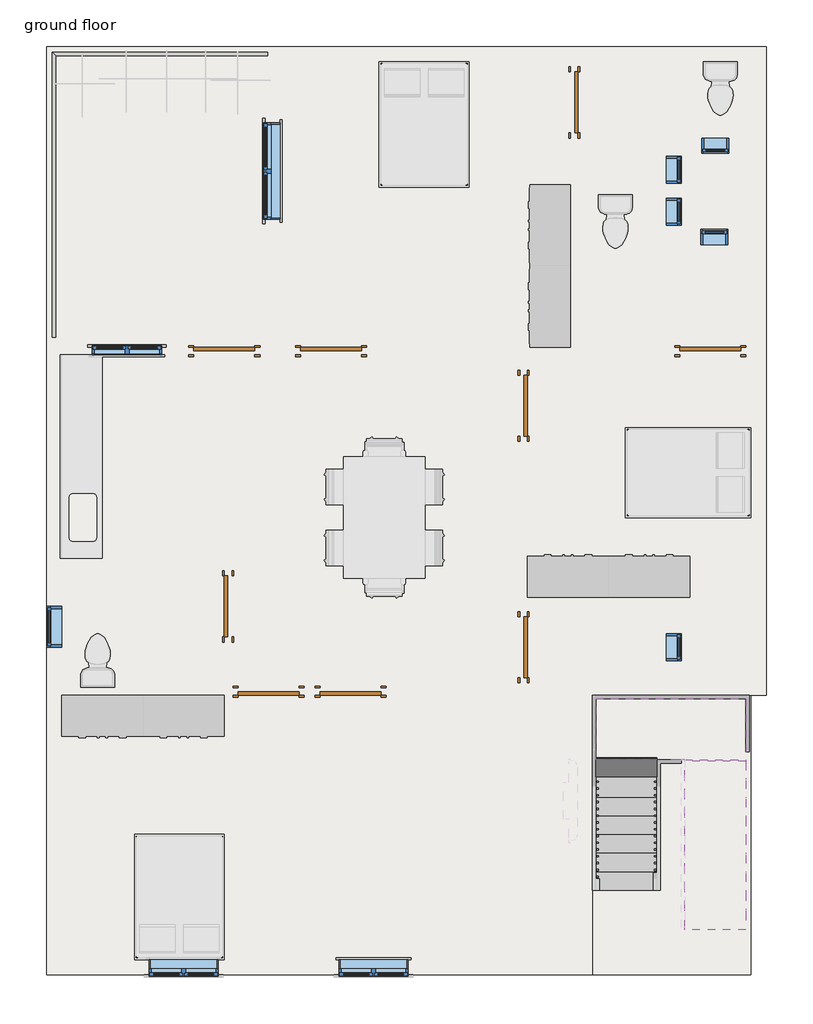
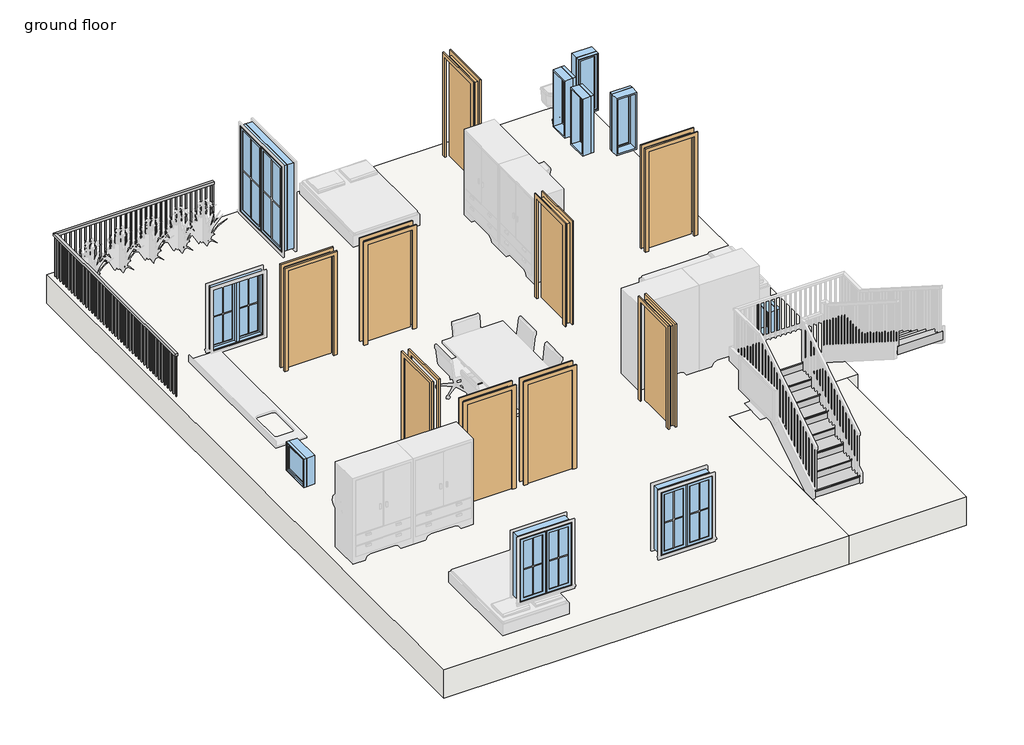
# One storey, part 1 of 3: 10 windows, 9 doors, 3 slabs, 2 stair flights, 1 railing.
"""IFC4 building model written with IfcOpenShell, lengths in millimetres."""

from ifc_helpers import new_model, si_unit, frame, origin, origin_with_axes, place, context, project, spatial, polyline, outline, extrude, faceted_brep, transform, mapped, element, save
from components import door_305aa2a5, door_e5f9f3c4, non_monolithic_landing_cf1353f8, stair_flight_d2e0b81c, stair_flight_50bec54b, window_aa618e30, window_cea7027f, window_80340324, window_8ddb865a, window_c95ebb39, window_9ac97e1a

model = new_model("IFC4")

# Units and contexts
model_context = context("Model", 3, world=origin())
ifc_project = project(units=[si_unit("LENGTHUNIT", "METRE", prefix="MILLI")], contexts=[model_context])

# Site, building, storey
site = spatial("IfcSite", under=ifc_project)
building = spatial("IfcBuilding", under=site)
storey = spatial("IfcBuildingStorey", under=building, Name="ground floor", Elevation=609.6)

# Doors
placement = place(None, origin())
door_shape = door_305aa2a5(model_context)
element("IfcDoor", 1, ObjectType="Single-Flush : 36\" x 84\"", at=placement, inside=storey, context=model_context, shape_type="MappedRepresentation", body=[
    mapped(door_shape, transform((-191.8998597, 11968.6257925, 609.6), x_axis=(0.0, 1.0, 0.0), y_axis=(-1.0, 0.0, 0.0), z_axis=(0.0, 0.0, 1.0))),
])
element("IfcDoor", 2, ObjectType="Single-Flush : 36\" x 84\"", at=placement, inside=storey, context=model_context, shape_type="MappedRepresentation", body=[
    mapped(door_shape, transform((-3843.1498597, 8241.1757925, 609.6), x_axis=(-1.0, 0.0, 0.0), y_axis=(0.0, -1.0, 0.0), z_axis=(0.0, 0.0, 1.0))),
])
element("IfcDoor", 3, ObjectType="Single-Flush : 36\" x 84\"", at=placement, inside=storey, context=model_context, shape_type="MappedRepresentation", body=[
    mapped(door_shape, transform((-953.8998597, 7422.0257925, 609.6), x_axis=(0.0, 1.0, 0.0), y_axis=(-1.0, 0.0, 0.0), z_axis=(0.0, 0.0, 1.0))),
])
element("IfcDoor", 4, ObjectType="Single-Flush : 36\" x 84\"", at=placement, inside=storey, context=model_context, shape_type="MappedRepresentation", body=[
    mapped(door_shape, transform((-4776.5998597, 3135.7757925, 609.6), x_axis=(1.0, 0.0, 0.0), y_axis=(0.0, 1.0, 0.0), z_axis=(0.0, 0.0, 1.0))),
])
door_2_shape = door_e5f9f3c4(model_context)
element("IfcDoor", 5, ObjectType="Single-Flush : 36\" x 84\"", at=placement, inside=storey, context=model_context, shape_type="MappedRepresentation", body=[
    mapped(door_2_shape, transform((1846.4501403, 8241.1757925, 609.6), x_axis=(1.0, 0.0, 0.0), y_axis=(0.0, 1.0, 0.0), z_axis=(0.0, 0.0, 1.0))),
])
element("IfcDoor", 6, ObjectType="Single-Flush : 36\" x 84\"", at=placement, inside=storey, context=model_context, shape_type="MappedRepresentation", body=[
    mapped(door_2_shape, transform((-5386.1998597, 4412.1257925, 609.6), x_axis=(0.0, 1.0, 0.0), y_axis=(-1.0, 0.0, 0.0), z_axis=(0.0, 0.0, 1.0))),
])
element("IfcDoor", 7, ObjectType="Single-Flush : 36\" x 84\"", at=placement, inside=storey, context=model_context, shape_type="MappedRepresentation", body=[
    mapped(door_2_shape, transform((-3551.0498597, 3135.7757925, 609.6), x_axis=(-1.0, 0.0, 0.0), y_axis=(0.0, -1.0, 0.0), z_axis=(0.0, 0.0, 1.0))),
])
element("IfcDoor", 8, ObjectType="Single-Flush : 36\" x 84\"", at=placement, inside=storey, context=model_context, shape_type="MappedRepresentation", body=[
    mapped(door_2_shape, transform((-953.8998597, 3802.5257925, 609.6), x_axis=(0.0, -1.0, 0.0), y_axis=(1.0, 0.0, 0.0), z_axis=(0.0, 0.0, 1.0))),
])
element("IfcDoor", 9, ObjectType="Single-Flush : 36\" x 84\"", at=placement, inside=storey, context=model_context, shape_type="MappedRepresentation", body=[
    mapped(door_2_shape, transform((-5443.3498597, 8241.1757925, 609.6), x_axis=(1.0, 0.0, 0.0), y_axis=(0.0, 1.0, 0.0), z_axis=(0.0, 0.0, 1.0))),
])

# Railing
element("IfcRailing", 10, ObjectType="Handrail - Rectangular", at=placement, inside=storey, context=model_context, shape_type="SolidModel", body=[
    faceted_brep([(-8021.4498597, 8450.7257925, 1524.0), (-8021.4498597, 8450.7257925, 1473.2), (-7970.6498597, 8450.7257925, 1473.2), (-7970.6498597, 8450.7257925, 1524.0), (-8021.4498597, 12717.9257925, 1524.0), (-8021.4498597, 12717.9257925, 1473.2), (-7970.6498597, 12667.1257925, 1473.2), (-7970.6498597, 12667.1257925, 1524.0), (-4795.6498597, 12717.9257925, 1524.0), (-4795.6498597, 12667.1257925, 1524.0), (-4795.6498597, 12667.1257925, 1473.2), (-4795.6498597, 12717.9257925, 1473.2)], [[[0, 1, 2, 3]], [[1, 0, 4, 5]], [[2, 1, 5, 6]], [[3, 2, 6, 7]], [[0, 3, 7, 4]], [[8, 9, 10, 11]], [[5, 4, 8, 11]], [[6, 5, 11, 10]], [[7, 6, 10, 9]], [[4, 7, 9, 8]]]),
    extrude(outline(polyline([(-4855.9748597, 12683.0007925), (-4855.9748597, 12702.0507925), (-4836.9248597, 12702.0507925), (-4836.9248597, 12683.0007925), (-4855.9748597, 12683.0007925)])), frame((0.0, 0.0, 609.6), z_axis=(0.0, 0.0, 1.0), x_axis=(1.0, 0.0, 0.0)), (0.0, 0.0, 1.0), 863.6),
    extrude(outline(polyline([(-4957.5748597, 12683.0007925), (-4957.5748597, 12702.0507925), (-4938.5248597, 12702.0507925), (-4938.5248597, 12683.0007925), (-4957.5748597, 12683.0007925)])), frame((0.0, 0.0, 609.6), z_axis=(0.0, 0.0, 1.0), x_axis=(1.0, 0.0, 0.0)), (0.0, 0.0, 1.0), 863.6),
    extrude(outline(polyline([(-5059.1748597, 12683.0007925), (-5059.1748597, 12702.0507925), (-5040.1248597, 12702.0507925), (-5040.1248597, 12683.0007925), (-5059.1748597, 12683.0007925)])), frame((0.0, 0.0, 609.6), z_axis=(0.0, 0.0, 1.0), x_axis=(1.0, 0.0, 0.0)), (0.0, 0.0, 1.0), 863.6),
    extrude(outline(polyline([(-5160.7748597, 12683.0007925), (-5160.7748597, 12702.0507925), (-5141.7248597, 12702.0507925), (-5141.7248597, 12683.0007925), (-5160.7748597, 12683.0007925)])), frame((0.0, 0.0, 609.6), z_axis=(0.0, 0.0, 1.0), x_axis=(1.0, 0.0, 0.0)), (0.0, 0.0, 1.0), 863.6),
    extrude(outline(polyline([(-5262.3748597, 12683.0007925), (-5262.3748597, 12702.0507925), (-5243.3248597, 12702.0507925), (-5243.3248597, 12683.0007925), (-5262.3748597, 12683.0007925)])), frame((0.0, 0.0, 609.6), z_axis=(0.0, 0.0, 1.0), x_axis=(1.0, 0.0, 0.0)), (0.0, 0.0, 1.0), 863.6),
    extrude(outline(polyline([(-5363.9748597, 12683.0007925), (-5363.9748597, 12702.0507925), (-5344.9248597, 12702.0507925), (-5344.9248597, 12683.0007925), (-5363.9748597, 12683.0007925)])), frame((0.0, 0.0, 609.6), z_axis=(0.0, 0.0, 1.0), x_axis=(1.0, 0.0, 0.0)), (0.0, 0.0, 1.0), 863.6),
    extrude(outline(polyline([(-5465.5748597, 12683.0007925), (-5465.5748597, 12702.0507925), (-5446.5248597, 12702.0507925), (-5446.5248597, 12683.0007925), (-5465.5748597, 12683.0007925)])), frame((0.0, 0.0, 609.6), z_axis=(0.0, 0.0, 1.0), x_axis=(1.0, 0.0, 0.0)), (0.0, 0.0, 1.0), 863.6),
    extrude(outline(polyline([(-5567.1748597, 12683.0007925), (-5567.1748597, 12702.0507925), (-5548.1248597, 12702.0507925), (-5548.1248597, 12683.0007925), (-5567.1748597, 12683.0007925)])), frame((0.0, 0.0, 609.6), z_axis=(0.0, 0.0, 1.0), x_axis=(1.0, 0.0, 0.0)), (0.0, 0.0, 1.0), 863.6),
    extrude(outline(polyline([(-5668.7748597, 12683.0007925), (-5668.7748597, 12702.0507925), (-5649.7248597, 12702.0507925), (-5649.7248597, 12683.0007925), (-5668.7748597, 12683.0007925)])), frame((0.0, 0.0, 609.6), z_axis=(0.0, 0.0, 1.0), x_axis=(1.0, 0.0, 0.0)), (0.0, 0.0, 1.0), 863.6),
    extrude(outline(polyline([(-5770.3748597, 12683.0007925), (-5770.3748597, 12702.0507925), (-5751.3248597, 12702.0507925), (-5751.3248597, 12683.0007925), (-5770.3748597, 12683.0007925)])), frame((0.0, 0.0, 609.6), z_axis=(0.0, 0.0, 1.0), x_axis=(1.0, 0.0, 0.0)), (0.0, 0.0, 1.0), 863.6),
    extrude(outline(polyline([(-5871.9748597, 12683.0007925), (-5871.9748597, 12702.0507925), (-5852.9248597, 12702.0507925), (-5852.9248597, 12683.0007925), (-5871.9748597, 12683.0007925)])), frame((0.0, 0.0, 609.6), z_axis=(0.0, 0.0, 1.0), x_axis=(1.0, 0.0, 0.0)), (0.0, 0.0, 1.0), 863.6),
    extrude(outline(polyline([(-5973.5748597, 12683.0007925), (-5973.5748597, 12702.0507925), (-5954.5248597, 12702.0507925), (-5954.5248597, 12683.0007925), (-5973.5748597, 12683.0007925)])), frame((0.0, 0.0, 609.6), z_axis=(0.0, 0.0, 1.0), x_axis=(1.0, 0.0, 0.0)), (0.0, 0.0, 1.0), 863.6),
    extrude(outline(polyline([(-6075.1748597, 12683.0007925), (-6075.1748597, 12702.0507925), (-6056.1248597, 12702.0507925), (-6056.1248597, 12683.0007925), (-6075.1748597, 12683.0007925)])), frame((0.0, 0.0, 609.6), z_axis=(0.0, 0.0, 1.0), x_axis=(1.0, 0.0, 0.0)), (0.0, 0.0, 1.0), 863.6),
    extrude(outline(polyline([(-6176.7748597, 12683.0007925), (-6176.7748597, 12702.0507925), (-6157.7248597, 12702.0507925), (-6157.7248597, 12683.0007925), (-6176.7748597, 12683.0007925)])), frame((0.0, 0.0, 609.6), z_axis=(0.0, 0.0, 1.0), x_axis=(1.0, 0.0, 0.0)), (0.0, 0.0, 1.0), 863.6),
    extrude(outline(polyline([(-6278.3748597, 12683.0007925), (-6278.3748597, 12702.0507925), (-6259.3248597, 12702.0507925), (-6259.3248597, 12683.0007925), (-6278.3748597, 12683.0007925)])), frame((0.0, 0.0, 609.6), z_axis=(0.0, 0.0, 1.0), x_axis=(1.0, 0.0, 0.0)), (0.0, 0.0, 1.0), 863.6),
    extrude(outline(polyline([(-6379.9748597, 12683.0007925), (-6379.9748597, 12702.0507925), (-6360.9248597, 12702.0507925), (-6360.9248597, 12683.0007925), (-6379.9748597, 12683.0007925)])), frame((0.0, 0.0, 609.6), z_axis=(0.0, 0.0, 1.0), x_axis=(1.0, 0.0, 0.0)), (0.0, 0.0, 1.0), 863.6),
    extrude(outline(polyline([(-6481.5748597, 12683.0007925), (-6481.5748597, 12702.0507925), (-6462.5248597, 12702.0507925), (-6462.5248597, 12683.0007925), (-6481.5748597, 12683.0007925)])), frame((0.0, 0.0, 609.6), z_axis=(0.0, 0.0, 1.0), x_axis=(1.0, 0.0, 0.0)), (0.0, 0.0, 1.0), 863.6),
    extrude(outline(polyline([(-6583.1748597, 12683.0007925), (-6583.1748597, 12702.0507925), (-6564.1248597, 12702.0507925), (-6564.1248597, 12683.0007925), (-6583.1748597, 12683.0007925)])), frame((0.0, 0.0, 609.6), z_axis=(0.0, 0.0, 1.0), x_axis=(1.0, 0.0, 0.0)), (0.0, 0.0, 1.0), 863.6),
    extrude(outline(polyline([(-6684.7748597, 12683.0007925), (-6684.7748597, 12702.0507925), (-6665.7248597, 12702.0507925), (-6665.7248597, 12683.0007925), (-6684.7748597, 12683.0007925)])), frame((0.0, 0.0, 609.6), z_axis=(0.0, 0.0, 1.0), x_axis=(1.0, 0.0, 0.0)), (0.0, 0.0, 1.0), 863.6),
    extrude(outline(polyline([(-6786.3748597, 12683.0007925), (-6786.3748597, 12702.0507925), (-6767.3248597, 12702.0507925), (-6767.3248597, 12683.0007925), (-6786.3748597, 12683.0007925)])), frame((0.0, 0.0, 609.6), z_axis=(0.0, 0.0, 1.0), x_axis=(1.0, 0.0, 0.0)), (0.0, 0.0, 1.0), 863.6),
    extrude(outline(polyline([(-6887.9748597, 12683.0007925), (-6887.9748597, 12702.0507925), (-6868.9248597, 12702.0507925), (-6868.9248597, 12683.0007925), (-6887.9748597, 12683.0007925)])), frame((0.0, 0.0, 609.6), z_axis=(0.0, 0.0, 1.0), x_axis=(1.0, 0.0, 0.0)), (0.0, 0.0, 1.0), 863.6),
    extrude(outline(polyline([(-6989.5748597, 12683.0007925), (-6989.5748597, 12702.0507925), (-6970.5248597, 12702.0507925), (-6970.5248597, 12683.0007925), (-6989.5748597, 12683.0007925)])), frame((0.0, 0.0, 609.6), z_axis=(0.0, 0.0, 1.0), x_axis=(1.0, 0.0, 0.0)), (0.0, 0.0, 1.0), 863.6),
    extrude(outline(polyline([(-7091.1748597, 12683.0007925), (-7091.1748597, 12702.0507925), (-7072.1248597, 12702.0507925), (-7072.1248597, 12683.0007925), (-7091.1748597, 12683.0007925)])), frame((0.0, 0.0, 609.6), z_axis=(0.0, 0.0, 1.0), x_axis=(1.0, 0.0, 0.0)), (0.0, 0.0, 1.0), 863.6),
    extrude(outline(polyline([(-7192.7748597, 12683.0007925), (-7192.7748597, 12702.0507925), (-7173.7248597, 12702.0507925), (-7173.7248597, 12683.0007925), (-7192.7748597, 12683.0007925)])), frame((0.0, 0.0, 609.6), z_axis=(0.0, 0.0, 1.0), x_axis=(1.0, 0.0, 0.0)), (0.0, 0.0, 1.0), 863.6),
    extrude(outline(polyline([(-7294.3748597, 12683.0007925), (-7294.3748597, 12702.0507925), (-7275.3248597, 12702.0507925), (-7275.3248597, 12683.0007925), (-7294.3748597, 12683.0007925)])), frame((0.0, 0.0, 609.6), z_axis=(0.0, 0.0, 1.0), x_axis=(1.0, 0.0, 0.0)), (0.0, 0.0, 1.0), 863.6),
    extrude(outline(polyline([(-7395.9748597, 12683.0007925), (-7395.9748597, 12702.0507925), (-7376.9248597, 12702.0507925), (-7376.9248597, 12683.0007925), (-7395.9748597, 12683.0007925)])), frame((0.0, 0.0, 609.6), z_axis=(0.0, 0.0, 1.0), x_axis=(1.0, 0.0, 0.0)), (0.0, 0.0, 1.0), 863.6),
    extrude(outline(polyline([(-7497.5748597, 12683.0007925), (-7497.5748597, 12702.0507925), (-7478.5248597, 12702.0507925), (-7478.5248597, 12683.0007925), (-7497.5748597, 12683.0007925)])), frame((0.0, 0.0, 609.6), z_axis=(0.0, 0.0, 1.0), x_axis=(1.0, 0.0, 0.0)), (0.0, 0.0, 1.0), 863.6),
    extrude(outline(polyline([(-7599.1748597, 12683.0007925), (-7599.1748597, 12702.0507925), (-7580.1248597, 12702.0507925), (-7580.1248597, 12683.0007925), (-7599.1748597, 12683.0007925)])), frame((0.0, 0.0, 609.6), z_axis=(0.0, 0.0, 1.0), x_axis=(1.0, 0.0, 0.0)), (0.0, 0.0, 1.0), 863.6),
    extrude(outline(polyline([(-7700.7748597, 12683.0007925), (-7700.7748597, 12702.0507925), (-7681.7248597, 12702.0507925), (-7681.7248597, 12683.0007925), (-7700.7748597, 12683.0007925)])), frame((0.0, 0.0, 609.6), z_axis=(0.0, 0.0, 1.0), x_axis=(1.0, 0.0, 0.0)), (0.0, 0.0, 1.0), 863.6),
    extrude(outline(polyline([(-7802.3748597, 12683.0007925), (-7802.3748597, 12702.0507925), (-7783.3248597, 12702.0507925), (-7783.3248597, 12683.0007925), (-7802.3748597, 12683.0007925)])), frame((0.0, 0.0, 609.6), z_axis=(0.0, 0.0, 1.0), x_axis=(1.0, 0.0, 0.0)), (0.0, 0.0, 1.0), 863.6),
    extrude(outline(polyline([(-7903.9748597, 12683.0007925), (-7903.9748597, 12702.0507925), (-7884.9248597, 12702.0507925), (-7884.9248597, 12683.0007925), (-7903.9748597, 12683.0007925)])), frame((0.0, 0.0, 609.6), z_axis=(0.0, 0.0, 1.0), x_axis=(1.0, 0.0, 0.0)), (0.0, 0.0, 1.0), 863.6),
    extrude(outline(polyline([(-7986.5248597, 12606.8007925), (-8005.5748597, 12606.8007925), (-8005.5748597, 12625.8507925), (-7986.5248597, 12625.8507925), (-7986.5248597, 12606.8007925)])), frame((0.0, 0.0, 609.6), z_axis=(0.0, 0.0, 1.0), x_axis=(1.0, 0.0, 0.0)), (0.0, 0.0, 1.0), 863.6),
    extrude(outline(polyline([(-7986.5248597, 12505.2007925), (-8005.5748597, 12505.2007925), (-8005.5748597, 12524.2507925), (-7986.5248597, 12524.2507925), (-7986.5248597, 12505.2007925)])), frame((0.0, 0.0, 609.6), z_axis=(0.0, 0.0, 1.0), x_axis=(1.0, 0.0, 0.0)), (0.0, 0.0, 1.0), 863.6),
    extrude(outline(polyline([(-7986.5248597, 12403.6007925), (-8005.5748597, 12403.6007925), (-8005.5748597, 12422.6507925), (-7986.5248597, 12422.6507925), (-7986.5248597, 12403.6007925)])), frame((0.0, 0.0, 609.6), z_axis=(0.0, 0.0, 1.0), x_axis=(1.0, 0.0, 0.0)), (0.0, 0.0, 1.0), 863.6),
    extrude(outline(polyline([(-7986.5248597, 12302.0007925), (-8005.5748597, 12302.0007925), (-8005.5748597, 12321.0507925), (-7986.5248597, 12321.0507925), (-7986.5248597, 12302.0007925)])), frame((0.0, 0.0, 609.6), z_axis=(0.0, 0.0, 1.0), x_axis=(1.0, 0.0, 0.0)), (0.0, 0.0, 1.0), 863.6),
    extrude(outline(polyline([(-7986.5248597, 12200.4007925), (-8005.5748597, 12200.4007925), (-8005.5748597, 12219.4507925), (-7986.5248597, 12219.4507925), (-7986.5248597, 12200.4007925)])), frame((0.0, 0.0, 609.6), z_axis=(0.0, 0.0, 1.0), x_axis=(1.0, 0.0, 0.0)), (0.0, 0.0, 1.0), 863.6),
    extrude(outline(polyline([(-7986.5248597, 12098.8007925), (-8005.5748597, 12098.8007925), (-8005.5748597, 12117.8507925), (-7986.5248597, 12117.8507925), (-7986.5248597, 12098.8007925)])), frame((0.0, 0.0, 609.6), z_axis=(0.0, 0.0, 1.0), x_axis=(1.0, 0.0, 0.0)), (0.0, 0.0, 1.0), 863.6),
    extrude(outline(polyline([(-7986.5248597, 11997.2007925), (-8005.5748597, 11997.2007925), (-8005.5748597, 12016.2507925), (-7986.5248597, 12016.2507925), (-7986.5248597, 11997.2007925)])), frame((0.0, 0.0, 609.6), z_axis=(0.0, 0.0, 1.0), x_axis=(1.0, 0.0, 0.0)), (0.0, 0.0, 1.0), 863.6),
    extrude(outline(polyline([(-7986.5248597, 11895.6007925), (-8005.5748597, 11895.6007925), (-8005.5748597, 11914.6507925), (-7986.5248597, 11914.6507925), (-7986.5248597, 11895.6007925)])), frame((0.0, 0.0, 609.6), z_axis=(0.0, 0.0, 1.0), x_axis=(1.0, 0.0, 0.0)), (0.0, 0.0, 1.0), 863.6),
    extrude(outline(polyline([(-7986.5248597, 11794.0007925), (-8005.5748597, 11794.0007925), (-8005.5748597, 11813.0507925), (-7986.5248597, 11813.0507925), (-7986.5248597, 11794.0007925)])), frame((0.0, 0.0, 609.6), z_axis=(0.0, 0.0, 1.0), x_axis=(1.0, 0.0, 0.0)), (0.0, 0.0, 1.0), 863.6),
    extrude(outline(polyline([(-7986.5248597, 11692.4007925), (-8005.5748597, 11692.4007925), (-8005.5748597, 11711.4507925), (-7986.5248597, 11711.4507925), (-7986.5248597, 11692.4007925)])), frame((0.0, 0.0, 609.6), z_axis=(0.0, 0.0, 1.0), x_axis=(1.0, 0.0, 0.0)), (0.0, 0.0, 1.0), 863.6),
    extrude(outline(polyline([(-7986.5248597, 11590.8007925), (-8005.5748597, 11590.8007925), (-8005.5748597, 11609.8507925), (-7986.5248597, 11609.8507925), (-7986.5248597, 11590.8007925)])), frame((0.0, 0.0, 609.6), z_axis=(0.0, 0.0, 1.0), x_axis=(1.0, 0.0, 0.0)), (0.0, 0.0, 1.0), 863.6),
    extrude(outline(polyline([(-7986.5248597, 11489.2007925), (-8005.5748597, 11489.2007925), (-8005.5748597, 11508.2507925), (-7986.5248597, 11508.2507925), (-7986.5248597, 11489.2007925)])), frame((0.0, 0.0, 609.6), z_axis=(0.0, 0.0, 1.0), x_axis=(1.0, 0.0, 0.0)), (0.0, 0.0, 1.0), 863.6),
    extrude(outline(polyline([(-7986.5248597, 11387.6007925), (-8005.5748597, 11387.6007925), (-8005.5748597, 11406.6507925), (-7986.5248597, 11406.6507925), (-7986.5248597, 11387.6007925)])), frame((0.0, 0.0, 609.6), z_axis=(0.0, 0.0, 1.0), x_axis=(1.0, 0.0, 0.0)), (0.0, 0.0, 1.0), 863.6),
    extrude(outline(polyline([(-7986.5248597, 11286.0007925), (-8005.5748597, 11286.0007925), (-8005.5748597, 11305.0507925), (-7986.5248597, 11305.0507925), (-7986.5248597, 11286.0007925)])), frame((0.0, 0.0, 609.6), z_axis=(0.0, 0.0, 1.0), x_axis=(1.0, 0.0, 0.0)), (0.0, 0.0, 1.0), 863.6),
    extrude(outline(polyline([(-7986.5248597, 11184.4007925), (-8005.5748597, 11184.4007925), (-8005.5748597, 11203.4507925), (-7986.5248597, 11203.4507925), (-7986.5248597, 11184.4007925)])), frame((0.0, 0.0, 609.6), z_axis=(0.0, 0.0, 1.0), x_axis=(1.0, 0.0, 0.0)), (0.0, 0.0, 1.0), 863.6),
    extrude(outline(polyline([(-7986.5248597, 11082.8007925), (-8005.5748597, 11082.8007925), (-8005.5748597, 11101.8507925), (-7986.5248597, 11101.8507925), (-7986.5248597, 11082.8007925)])), frame((0.0, 0.0, 609.6), z_axis=(0.0, 0.0, 1.0), x_axis=(1.0, 0.0, 0.0)), (0.0, 0.0, 1.0), 863.6),
    extrude(outline(polyline([(-7986.5248597, 10981.2007925), (-8005.5748597, 10981.2007925), (-8005.5748597, 11000.2507925), (-7986.5248597, 11000.2507925), (-7986.5248597, 10981.2007925)])), frame((0.0, 0.0, 609.6), z_axis=(0.0, 0.0, 1.0), x_axis=(1.0, 0.0, 0.0)), (0.0, 0.0, 1.0), 863.6),
    extrude(outline(polyline([(-7986.5248597, 10879.6007925), (-8005.5748597, 10879.6007925), (-8005.5748597, 10898.6507925), (-7986.5248597, 10898.6507925), (-7986.5248597, 10879.6007925)])), frame((0.0, 0.0, 609.6), z_axis=(0.0, 0.0, 1.0), x_axis=(1.0, 0.0, 0.0)), (0.0, 0.0, 1.0), 863.6),
    extrude(outline(polyline([(-7986.5248597, 10778.0007925), (-8005.5748597, 10778.0007925), (-8005.5748597, 10797.0507925), (-7986.5248597, 10797.0507925), (-7986.5248597, 10778.0007925)])), frame((0.0, 0.0, 609.6), z_axis=(0.0, 0.0, 1.0), x_axis=(1.0, 0.0, 0.0)), (0.0, 0.0, 1.0), 863.6),
    extrude(outline(polyline([(-7986.5248597, 10676.4007925), (-8005.5748597, 10676.4007925), (-8005.5748597, 10695.4507925), (-7986.5248597, 10695.4507925), (-7986.5248597, 10676.4007925)])), frame((0.0, 0.0, 609.6), z_axis=(0.0, 0.0, 1.0), x_axis=(1.0, 0.0, 0.0)), (0.0, 0.0, 1.0), 863.6),
    extrude(outline(polyline([(-7986.5248597, 10574.8007925), (-8005.5748597, 10574.8007925), (-8005.5748597, 10593.8507925), (-7986.5248597, 10593.8507925), (-7986.5248597, 10574.8007925)])), frame((0.0, 0.0, 609.6), z_axis=(0.0, 0.0, 1.0), x_axis=(1.0, 0.0, 0.0)), (0.0, 0.0, 1.0), 863.6),
    extrude(outline(polyline([(-7986.5248597, 10473.2007925), (-8005.5748597, 10473.2007925), (-8005.5748597, 10492.2507925), (-7986.5248597, 10492.2507925), (-7986.5248597, 10473.2007925)])), frame((0.0, 0.0, 609.6), z_axis=(0.0, 0.0, 1.0), x_axis=(1.0, 0.0, 0.0)), (0.0, 0.0, 1.0), 863.6),
    extrude(outline(polyline([(-7986.5248597, 10371.6007925), (-8005.5748597, 10371.6007925), (-8005.5748597, 10390.6507925), (-7986.5248597, 10390.6507925), (-7986.5248597, 10371.6007925)])), frame((0.0, 0.0, 609.6), z_axis=(0.0, 0.0, 1.0), x_axis=(1.0, 0.0, 0.0)), (0.0, 0.0, 1.0), 863.6),
    extrude(outline(polyline([(-7986.5248597, 10270.0007925), (-8005.5748597, 10270.0007925), (-8005.5748597, 10289.0507925), (-7986.5248597, 10289.0507925), (-7986.5248597, 10270.0007925)])), frame((0.0, 0.0, 609.6), z_axis=(0.0, 0.0, 1.0), x_axis=(1.0, 0.0, 0.0)), (0.0, 0.0, 1.0), 863.6),
    extrude(outline(polyline([(-7986.5248597, 10168.4007925), (-8005.5748597, 10168.4007925), (-8005.5748597, 10187.4507925), (-7986.5248597, 10187.4507925), (-7986.5248597, 10168.4007925)])), frame((0.0, 0.0, 609.6), z_axis=(0.0, 0.0, 1.0), x_axis=(1.0, 0.0, 0.0)), (0.0, 0.0, 1.0), 863.6),
    extrude(outline(polyline([(-7986.5248597, 10066.8007925), (-8005.5748597, 10066.8007925), (-8005.5748597, 10085.8507925), (-7986.5248597, 10085.8507925), (-7986.5248597, 10066.8007925)])), frame((0.0, 0.0, 609.6), z_axis=(0.0, 0.0, 1.0), x_axis=(1.0, 0.0, 0.0)), (0.0, 0.0, 1.0), 863.6),
    extrude(outline(polyline([(-7986.5248597, 9965.2007925), (-8005.5748597, 9965.2007925), (-8005.5748597, 9984.2507925), (-7986.5248597, 9984.2507925), (-7986.5248597, 9965.2007925)])), frame((0.0, 0.0, 609.6), z_axis=(0.0, 0.0, 1.0), x_axis=(1.0, 0.0, 0.0)), (0.0, 0.0, 1.0), 863.6),
    extrude(outline(polyline([(-7986.5248597, 9863.6007925), (-8005.5748597, 9863.6007925), (-8005.5748597, 9882.6507925), (-7986.5248597, 9882.6507925), (-7986.5248597, 9863.6007925)])), frame((0.0, 0.0, 609.6), z_axis=(0.0, 0.0, 1.0), x_axis=(1.0, 0.0, 0.0)), (0.0, 0.0, 1.0), 863.6),
    extrude(outline(polyline([(-7986.5248597, 9762.0007925), (-8005.5748597, 9762.0007925), (-8005.5748597, 9781.0507925), (-7986.5248597, 9781.0507925), (-7986.5248597, 9762.0007925)])), frame((0.0, 0.0, 609.6), z_axis=(0.0, 0.0, 1.0), x_axis=(1.0, 0.0, 0.0)), (0.0, 0.0, 1.0), 863.6),
    extrude(outline(polyline([(-7986.5248597, 9660.4007925), (-8005.5748597, 9660.4007925), (-8005.5748597, 9679.4507925), (-7986.5248597, 9679.4507925), (-7986.5248597, 9660.4007925)])), frame((0.0, 0.0, 609.6), z_axis=(0.0, 0.0, 1.0), x_axis=(1.0, 0.0, 0.0)), (0.0, 0.0, 1.0), 863.6),
    extrude(outline(polyline([(-7986.5248597, 9558.8007925), (-8005.5748597, 9558.8007925), (-8005.5748597, 9577.8507925), (-7986.5248597, 9577.8507925), (-7986.5248597, 9558.8007925)])), frame((0.0, 0.0, 609.6), z_axis=(0.0, 0.0, 1.0), x_axis=(1.0, 0.0, 0.0)), (0.0, 0.0, 1.0), 863.6),
    extrude(outline(polyline([(-7986.5248597, 9457.2007925), (-8005.5748597, 9457.2007925), (-8005.5748597, 9476.2507925), (-7986.5248597, 9476.2507925), (-7986.5248597, 9457.2007925)])), frame((0.0, 0.0, 609.6), z_axis=(0.0, 0.0, 1.0), x_axis=(1.0, 0.0, 0.0)), (0.0, 0.0, 1.0), 863.6),
    extrude(outline(polyline([(-7986.5248597, 9355.6007925), (-8005.5748597, 9355.6007925), (-8005.5748597, 9374.6507925), (-7986.5248597, 9374.6507925), (-7986.5248597, 9355.6007925)])), frame((0.0, 0.0, 609.6), z_axis=(0.0, 0.0, 1.0), x_axis=(1.0, 0.0, 0.0)), (0.0, 0.0, 1.0), 863.6),
    extrude(outline(polyline([(-7986.5248597, 9254.0007925), (-8005.5748597, 9254.0007925), (-8005.5748597, 9273.0507925), (-7986.5248597, 9273.0507925), (-7986.5248597, 9254.0007925)])), frame((0.0, 0.0, 609.6), z_axis=(0.0, 0.0, 1.0), x_axis=(1.0, 0.0, 0.0)), (0.0, 0.0, 1.0), 863.6),
    extrude(outline(polyline([(-7986.5248597, 9152.4007925), (-8005.5748597, 9152.4007925), (-8005.5748597, 9171.4507925), (-7986.5248597, 9171.4507925), (-7986.5248597, 9152.4007925)])), frame((0.0, 0.0, 609.6), z_axis=(0.0, 0.0, 1.0), x_axis=(1.0, 0.0, 0.0)), (0.0, 0.0, 1.0), 863.6),
    extrude(outline(polyline([(-7986.5248597, 9050.8007925), (-8005.5748597, 9050.8007925), (-8005.5748597, 9069.8507925), (-7986.5248597, 9069.8507925), (-7986.5248597, 9050.8007925)])), frame((0.0, 0.0, 609.6), z_axis=(0.0, 0.0, 1.0), x_axis=(1.0, 0.0, 0.0)), (0.0, 0.0, 1.0), 863.6),
    extrude(outline(polyline([(-7986.5248597, 8949.2007925), (-8005.5748597, 8949.2007925), (-8005.5748597, 8968.2507925), (-7986.5248597, 8968.2507925), (-7986.5248597, 8949.2007925)])), frame((0.0, 0.0, 609.6), z_axis=(0.0, 0.0, 1.0), x_axis=(1.0, 0.0, 0.0)), (0.0, 0.0, 1.0), 863.6),
    extrude(outline(polyline([(-7986.5248597, 8847.6007925), (-8005.5748597, 8847.6007925), (-8005.5748597, 8866.6507925), (-7986.5248597, 8866.6507925), (-7986.5248597, 8847.6007925)])), frame((0.0, 0.0, 609.6), z_axis=(0.0, 0.0, 1.0), x_axis=(1.0, 0.0, 0.0)), (0.0, 0.0, 1.0), 863.6),
    extrude(outline(polyline([(-7986.5248597, 8746.0007925), (-8005.5748597, 8746.0007925), (-8005.5748597, 8765.0507925), (-7986.5248597, 8765.0507925), (-7986.5248597, 8746.0007925)])), frame((0.0, 0.0, 609.6), z_axis=(0.0, 0.0, 1.0), x_axis=(1.0, 0.0, 0.0)), (0.0, 0.0, 1.0), 863.6),
    extrude(outline(polyline([(-7986.5248597, 8644.4007925), (-8005.5748597, 8644.4007925), (-8005.5748597, 8663.4507925), (-7986.5248597, 8663.4507925), (-7986.5248597, 8644.4007925)])), frame((0.0, 0.0, 609.6), z_axis=(0.0, 0.0, 1.0), x_axis=(1.0, 0.0, 0.0)), (0.0, 0.0, 1.0), 863.6),
    extrude(outline(polyline([(-7986.5248597, 8542.8007925), (-8005.5748597, 8542.8007925), (-8005.5748597, 8561.8507925), (-7986.5248597, 8561.8507925), (-7986.5248597, 8542.8007925)])), frame((0.0, 0.0, 609.6), z_axis=(0.0, 0.0, 1.0), x_axis=(1.0, 0.0, 0.0)), (0.0, 0.0, 1.0), 863.6),
    extrude(outline(polyline([(-7986.5248597, 12683.0007925), (-8005.5748597, 12683.0007925), (-8005.5748597, 12702.0507925), (-7986.5248597, 12702.0507925), (-7986.5248597, 12683.0007925)])), frame((0.0, 0.0, 609.6), z_axis=(0.0, 0.0, 1.0), x_axis=(1.0, 0.0, 0.0)), (0.0, 0.0, 1.0), 863.6),
    extrude(outline(polyline([(-4814.6998597, 12683.0007925), (-4814.6998597, 12702.0507925), (-4795.6498597, 12702.0507925), (-4795.6498597, 12683.0007925), (-4814.6998597, 12683.0007925)])), frame((0.0, 0.0, 609.6), z_axis=(0.0, 0.0, 1.0), x_axis=(1.0, 0.0, 0.0)), (0.0, 0.0, 1.0), 863.6),
    extrude(outline(polyline([(-7986.5248597, 8450.7257925), (-8005.5748597, 8450.7257925), (-8005.5748597, 8469.7757925), (-7986.5248597, 8469.7757925), (-7986.5248597, 8450.7257925)])), frame((0.0, 0.0, 609.6), z_axis=(0.0, 0.0, 1.0), x_axis=(1.0, 0.0, 0.0)), (0.0, 0.0, 1.0), 863.6),
])

# Slabs
non_monolithic_landing_shape = non_monolithic_landing_cf1353f8(model_context)
element("IfcSlab", 11, ObjectType="Non-Monolithic Landing", at=placement, inside=storey, context=model_context, shape_type="MappedRepresentation", body=[
    mapped(non_monolithic_landing_shape, transform((0.0, 0.0, 0.0), x_axis=(1.0, 0.0, 0.0), y_axis=(0.0, 1.0, 0.0), z_axis=(0.0, 0.0, 1.0))),
])
element("IfcSlab", 12, ObjectType="slab 2'", at=placement, inside=storey, context=model_context, shape_type="SweptSolid", body=[
    extrude(outline(polyline([(2684.6501403, 12806.8257925), (2684.6501403, 3078.6257925), (81.1501403, 3078.6257925), (81.1501403, -1112.3742075), (-8110.3498597, -1112.3742075), (-8110.3498597, 12806.8257925), (2684.6501403, 12806.8257925)])), origin_with_axes(), (0.0, 0.0, 1.0), 609.6),
])
element("IfcSlab", 13, ObjectType="slab 2'", at=placement, inside=storey, context=model_context, shape_type="SweptSolid", body=[
    extrude(outline(polyline([(2456.0501403, -1112.3742075), (81.1501403, -1112.3742075), (81.1501403, 3078.6257925), (2456.0501403, 3078.6257925), (2456.0501403, -1112.3742075)])), origin_with_axes(), (0.0, 0.0, 1.0), 609.6),
])

# Stair flights
stair_flight_shape = stair_flight_d2e0b81c(model_context)
element("IfcStairFlight", 14, ObjectType="2\" Tread 1\" Nosing 1/4\" Riser", at=placement, inside=storey, context=model_context, shape_type="MappedRepresentation", body=[
    mapped(stair_flight_shape, transform((0.0, 0.0, 0.0), x_axis=(1.0, 0.0, 0.0), y_axis=(0.0, 1.0, 0.0), z_axis=(0.0, 0.0, 1.0))),
])
stair_flight_2_shape = stair_flight_50bec54b(model_context)
element("IfcStairFlight", 15, ObjectType="2\" Tread 1\" Nosing 1/4\" Riser", at=placement, inside=storey, context=model_context, shape_type="MappedRepresentation", body=[
    mapped(stair_flight_2_shape, transform((0.0, 0.0, 0.0), x_axis=(1.0, 0.0, 0.0), y_axis=(0.0, 1.0, 0.0), z_axis=(0.0, 0.0, 1.0))),
])

# Windows
window_shape = window_aa618e30(model_context)
element("IfcWindow", 16, ObjectType="Fixed : 16\" x 24\"", at=placement, inside=storey, context=model_context, shape_type="MappedRepresentation", body=[
    mapped(window_shape, transform((1300.3501403, 3764.4257925, 609.6), x_axis=(0.0, -1.0, 0.0), y_axis=(1.0, 0.0, 0.0), z_axis=(0.0, 0.0, 1.0))),
])
window_2_shape = window_cea7027f(model_context)
element("IfcWindow", 17, ObjectType="Fixed : 16\" x 48\"", at=placement, inside=storey, context=model_context, shape_type="MappedRepresentation", body=[
    mapped(window_2_shape, transform((1948.0501403, 9949.3257925, 609.6), x_axis=(1.0, 0.0, 0.0), y_axis=(0.0, 1.0, 0.0), z_axis=(0.0, 0.0, 1.0))),
])
element("IfcWindow", 18, ObjectType="Fixed : 16\" x 48\"", at=placement, inside=storey, context=model_context, shape_type="MappedRepresentation", body=[
    mapped(window_2_shape, transform((1884.5501403, 11320.9257925, 609.6), x_axis=(-1.0, 0.0, 0.0), y_axis=(0.0, -1.0, 0.0), z_axis=(0.0, 0.0, 1.0))),
])
element("IfcWindow", 19, ObjectType="Fixed : 16\" x 48\"", at=placement, inside=storey, context=model_context, shape_type="MappedRepresentation", body=[
    mapped(window_2_shape, transform((1300.3501403, 10292.2257925, 609.6), x_axis=(0.0, -1.0, 0.0), y_axis=(1.0, 0.0, 0.0), z_axis=(0.0, 0.0, 1.0))),
])
element("IfcWindow", 20, ObjectType="Fixed : 16\" x 48\"", at=placement, inside=storey, context=model_context, shape_type="MappedRepresentation", body=[
    mapped(window_2_shape, transform((1300.3501403, 10920.8299127, 609.6), x_axis=(0.0, -1.0, 0.0), y_axis=(1.0, 0.0, 0.0), z_axis=(0.0, 0.0, 1.0))),
])
window_3_shape = window_80340324(model_context)
element("IfcWindow", 21, ObjectType="Fixed : 24\" x 24\"", at=placement, inside=storey, context=model_context, shape_type="MappedRepresentation", body=[
    mapped(window_3_shape, transform((-7996.0498597, 4145.4257925, 609.6), x_axis=(0.0, 1.0, 0.0), y_axis=(-1.0, 0.0, 0.0), z_axis=(0.0, 0.0, 1.0))),
])
window_4_shape = window_8ddb865a(model_context)
element("IfcWindow", 22, ObjectType="Window-Casement-Double : 41\" x 53\"", at=placement, inside=storey, context=model_context, shape_type="MappedRepresentation", body=[
    mapped(window_4_shape, transform((-6903.8498597, 8241.1757925, 609.6), x_axis=(1.0, 0.0, 0.0), y_axis=(0.0, 1.0, 0.0), z_axis=(0.0, 0.0, 1.0))),
])
window_5_shape = window_c95ebb39(model_context)
element("IfcWindow", 23, ObjectType="Window-Casement-Double : 41\" x 53\"", at=placement, inside=storey, context=model_context, shape_type="MappedRepresentation", body=[
    mapped(window_5_shape, transform((-6052.9498597, -998.0742075, 609.6), x_axis=(-1.0, 0.0, 0.0), y_axis=(0.0, -1.0, 0.0), z_axis=(0.0, 0.0, 1.0))),
])
element("IfcWindow", 24, ObjectType="Window-Casement-Double : 41\" x 53\"", at=placement, inside=storey, context=model_context, shape_type="MappedRepresentation", body=[
    mapped(window_5_shape, transform((-3204.8498597, -998.0742075, 609.6), x_axis=(-1.0, 0.0, 0.0), y_axis=(0.0, -1.0, 0.0), z_axis=(0.0, 0.0, 1.0))),
])
window_6_shape = window_9ac97e1a(model_context)
element("IfcWindow", 25, ObjectType="Window-Casement-Double : 57\" x 72\"", at=placement, inside=storey, context=model_context, shape_type="MappedRepresentation", body=[
    mapped(window_6_shape, transform((-4719.4498597, 10939.9257925, 609.6), x_axis=(0.0, 1.0, 0.0), y_axis=(-1.0, 0.0, 0.0), z_axis=(0.0, 0.0, 1.0))),
])

save(model, "model.ifc")

# Revit data of these elements
# Type "Single-Flush : 36\" x 84\""
#   Type Mark = "1"
#   Construction Type Id = "MDOOR"
#   Assembly Code = "C1020"
#   Analytic Construction = "Metal"
#   Thickness = 0' - 2"
#   Heat Transfer Coefficient (U) = 0.651978 BTU/(h·ft²·°F)
#   Height = 7' - 0"
#   Trim Projection Ext = 0' - 1"
#   Trim Projection Int = 0' - 1"
#   Trim Width = 0' - 3"
#   Width = 3' - 0"
#   Define Thermal Properties by = 1
#   Define Thermal Properties by = 1
#   Door Material = Door - Panel
#   Frame Material = Door - Frame
#   Visual Light Transmittance = 0
#   Solar Heat Gain Coefficient = 0
#   Function = (empty or 0)
#   Wall Closure = (empty or 0)
# Type "Handrail - Rectangular"
#   Assembly Code = "C2010400"
#   built-in parameter 1008612 = 0.0416667 (stored number, unit not read)
#   built-in parameter 1008611 = 0.0416667 (stored number, unit not read)
#   built-in parameter 1008609 = 0.333333 (stored number, unit not read)
#   built-in parameter 1008604 = 0.166667 (stored number, unit not read)
#   built-in parameter 1008603 = 0.166667 (stored number, unit not read)
#   Railing Height = 3' - 0"
#   built-in parameter 1008630 = 2
#   built-in parameter 1008610 = 2
#   built-in parameter 1008618 = Baluster - Square : 3/4"
# Type "slab 2'"
#   Assembly Code = "B1010"
#   Function = 0
#   Layers, outside or top first: 2' - 0" "Concrete, Cast-in-Place gray" (function 1)
# Type "Fixed : 16\" x 24\""
#   Type Mark = "4"
#   Construction Type Id = "GSP4R"
#   Assembly Code = "B2020100"
#   Analytic Construction = "1/8 in Pilkington single glazing"
#   Visual Light Transmittance = 0.9
#   Solar Heat Gain Coefficient = 0.78
#   Heat Transfer Coefficient (U) = 0.6496 BTU/(h·ft²·°F)
#   Height = 2' - 0"
#   Default Sill Height = 3' - 0"
#   Width = 1' - 4"
#   Window Inset = 0' - 0 3/4"
#   Define Thermal Properties by = 1
#   Define Thermal Properties by = 1
#   Glass Pane Material = Glass
#   Sash Material = Sash
#   Wall Closure = (empty or 0)
# Type "Fixed : 16\" x 48\""
#   Type Mark = "5"
#   Construction Type Id = "GSP4R"
#   Assembly Code = "B2020100"
#   Analytic Construction = "1/8 in Pilkington single glazing"
#   Visual Light Transmittance = 0.9
#   Solar Heat Gain Coefficient = 0.78
#   Heat Transfer Coefficient (U) = 0.6496 BTU/(h·ft²·°F)
#   Height = 4' - 0"
#   Default Sill Height = 3' - 0"
#   Width = 1' - 4"
#   Window Inset = 0' - 0 3/4"
#   Define Thermal Properties by = 1
#   Define Thermal Properties by = 1
#   Glass Pane Material = Glass
#   Sash Material = Sash
#   Wall Closure = (empty or 0)
# Type "Fixed : 24\" x 24\""
#   Type Mark = "3"
#   Construction Type Id = "GSP4R"
#   Assembly Code = "B2020100"
#   Analytic Construction = "1/8 in Pilkington single glazing"
#   Visual Light Transmittance = 0.9
#   Solar Heat Gain Coefficient = 0.78
#   Heat Transfer Coefficient (U) = 0.6496 BTU/(h·ft²·°F)
#   Height = 2' - 0"
#   Default Sill Height = 3' - 0"
#   Width = 2' - 0"
#   Window Inset = 0' - 0 3/4"
#   Define Thermal Properties by = 1
#   Define Thermal Properties by = 1
#   Glass Pane Material = Glass
#   Sash Material = Sash
#   Wall Closure = (empty or 0)
# Type "Window-Casement-Double : 41\" x 53\""
#   Type Mark = "15"
#   Fire Rating = "0.5h"
#   Assembly Code = "B2020100"
#   Analytic Construction = "Double glazing - domestic"
#   Frame Extension [instance default] = 0' - 0 1/4"
#   Window Inset [instance default] = 0' - 0"
#   Wall Thickness [instance default] = 0' - 6"
#   Interior Wall Closure [instance default] = 0' - 2 1/4"
#   Half Width = 1' - 8 1/2"
#   Visual Light Transmittance = 0.81
#   Thermal Resistance (R) = 1.8146 (h·ft²·°F)/BTU
#   Solar Heat Gain Coefficient = 0.76
#   Rough Width = 3' - 5 1/2"
#   Rough Height = 4' - 5 1/2"
#   Height = 4' - 5"
#   Heat Transfer Coefficient (U) = 0.5511 BTU/(h·ft²·°F)
#   Exterior Wall Closure [instance default] = 0' - 1 1/4"
#   Extension Jamb [instance default] = 0' - 2 1/4"
#   Default Sill Height = 3' - 0"
#   Width = 3' - 5"
#   Define Thermal Properties by = 0
#   Muntin Visibility = yes
#   Interior Trim Visibility [instance default] = yes
#   Exterior Trim Visibility [instance default] = yes
#   Extension Jamb Visibility [instance default] = yes
#   Interior Trim Material = Wood - Stained
#   Muntin Pattern = Muntin Pattern_2x2 : Muntin Pattern_2x2
#   Interior Trim = Trim-Window-Interior-Flat : Picture Frame
#   Interior Frame Material = Wood - Stained
#   Glass Panel Material = Glass
#   Exterior Trim Material = Clad - White
#   Exterior Trim = Trim-Window-Exterior-Flat : with Sill
#   Exterior Frame Material = Clad - White
#   Wall Closure = (empty or 0)
# Type "Window-Casement-Double : 57\" x 72\""
#   Type Mark = "17"
#   Fire Rating = "0.5h"
#   Assembly Code = "B2020100"
#   Analytic Construction = "Double glazing - domestic"
#   Frame Extension [instance default] = 0' - 0 1/4"
#   Window Inset [instance default] = 0' - 0"
#   Wall Thickness [instance default] = 0' - 6"
#   Interior Wall Closure [instance default] = 0' - 2 1/4"
#   Half Width = 2' - 4 1/2"
#   Visual Light Transmittance = 0.81
#   Thermal Resistance (R) = 1.8146 (h·ft²·°F)/BTU
#   Solar Heat Gain Coefficient = 0.76
#   Rough Width = 4' - 9 1/2"
#   Rough Height = 6' - 0 1/2"
#   Height = 6' - 0"
#   Heat Transfer Coefficient (U) = 0.5511 BTU/(h·ft²·°F)
#   Exterior Wall Closure [instance default] = 0' - 1 1/4"
#   Extension Jamb [instance default] = 0' - 2 1/4"
#   Default Sill Height = 3' - 0"
#   Width = 4' - 9"
#   Define Thermal Properties by = 0
#   Muntin Visibility = yes
#   Interior Trim Visibility [instance default] = yes
#   Exterior Trim Visibility [instance default] = yes
#   Extension Jamb Visibility [instance default] = yes
#   Interior Trim Material = Wood - Stained
#   Muntin Pattern = Muntin Pattern_2x2 : Muntin Pattern_2x2
#   Interior Trim = Trim-Window-Interior-Flat : Picture Frame
#   Interior Frame Material = Wood - Stained
#   Glass Panel Material = Glass
#   Exterior Trim Material = Clad - White
#   Exterior Trim = Trim-Window-Exterior-Flat : with Sill
#   Exterior Frame Material = Clad - White
#   Wall Closure = (empty or 0)
# Elements 1, 2, 3, 4, 5, 6, 7, 8, 9 (IfcDoor, "Single-Flush : 36\" x 84\"")
#   Phase Created = New Construction
#   Materials on its faces: "Door - Frame", "Door - Panel"
# Element 10 (IfcRailing, "Handrail - Rectangular")
#   Phase Created = New Construction
# Element 11 (IfcSlab, "Non-Monolithic Landing")
#   Phase Created = New Construction
# Elements 12, 13 (IfcSlab, "slab 2'")
#   Height Offset From Level = 0' - 0"
#   Phase Created = New Construction
#   Materials on its faces: "Concrete, Cast-in-Place gray"
# Elements 14, 15 (IfcStairFlight, "2\" Tread 1\" Nosing 1/4\" Riser")
#   Phase Created = New Construction
# Element 16 (IfcWindow, "Fixed : 16\" x 24\"")
#   Mark = "11"
#   Phase Created = New Construction
#   Materials on its faces: "Sash", "Glass"
# Element 17 (IfcWindow, "Fixed : 16\" x 48\"")
#   Mark = "7"
#   Phase Created = New Construction
#   Materials on its faces: "Sash", "Glass"
# Element 18 (IfcWindow, "Fixed : 16\" x 48\"")
#   Mark = "8"
#   Phase Created = New Construction
#   Materials on its faces: "Sash", "Glass"
# Element 19 (IfcWindow, "Fixed : 16\" x 48\"")
#   Mark = "13"
#   Phase Created = New Construction
#   Materials on its faces: "Sash", "Glass"
# Element 20 (IfcWindow, "Fixed : 16\" x 48\"")
#   Mark = "14"
#   Phase Created = New Construction
#   Materials on its faces: "Sash", "Glass"
# Element 21 (IfcWindow, "Fixed : 24\" x 24\"")
#   Mark = "12"
#   Phase Created = New Construction
#   Materials on its faces: "Sash", "Glass"
# Element 22 (IfcWindow, "Window-Casement-Double : 41\" x 53\"")
#   Mark = "2"
#   Window Inset = 0' - 0"
#   Interior Wall Closure = 0' - 2 1/4"
#   Frame Extension = 0' - 0 1/4"
#   Exterior Wall Closure = 0' - 1 1/4"
#   Interior Trim Visibility = yes
#   Exterior Trim Visibility = yes
#   Phase Created = New Construction
#   Materials on its faces: "Wood - Stained", "Glass", "Clad - White"
# Element 23 (IfcWindow, "Window-Casement-Double : 41\" x 53\"")
#   Mark = "3"
#   Window Inset = 0' - 0"
#   Interior Wall Closure = 0' - 2 1/4"
#   Frame Extension = 0' - 0 1/4"
#   Exterior Wall Closure = 0' - 1 1/4"
#   Interior Trim Visibility = yes
#   Exterior Trim Visibility = yes
#   Phase Created = New Construction
#   Materials on its faces: "Wood - Stained", "Glass", "Clad - White"
# Element 24 (IfcWindow, "Window-Casement-Double : 41\" x 53\"")
#   Mark = "4"
#   Window Inset = 0' - 0"
#   Interior Wall Closure = 0' - 2 1/4"
#   Frame Extension = 0' - 0 1/4"
#   Exterior Wall Closure = 0' - 1 1/4"
#   Interior Trim Visibility = yes
#   Exterior Trim Visibility = yes
#   Phase Created = New Construction
#   Materials on its faces: "Wood - Stained", "Glass", "Clad - White"
# Element 25 (IfcWindow, "Window-Casement-Double : 57\" x 72\"")
#   Mark = "1"
#   Window Inset = 0' - 0"
#   Interior Wall Closure = 0' - 2 1/4"
#   Frame Extension = 0' - 0 1/4"
#   Exterior Wall Closure = 0' - 1 1/4"
#   Interior Trim Visibility = yes
#   Exterior Trim Visibility = yes
#   Phase Created = New Construction
#   Materials on its faces: "Wood - Stained", "Glass", "Clad - White"
# Materials
#   "Door - Panel": class "Wood", colour RGB 210 159 95, transparency 0, Cost = 0
#   "Door - Frame": colour RGB 118 70 51, transparency 0, Cost = 0
#   "Concrete, Cast-in-Place gray": class "Concrete", colour RGB 192 192 192, transparency 0, Description = "Cast-in-place concrete", Cost = 0
#   "Glass": class "Glass", colour RGB 0 128 192, transparency 0.75, Description = "Soda Lime Glass", Cost = 0
#   "Sash": class "Wood", colour RGB 224 178 126, transparency 0, Cost = 0
#   "Wood - Stained": class "Wood", colour RGB 224 178 126, transparency 0, Cost = 0
#   "Clad - White": class "Wood", colour RGB 242 242 238, transparency 0, Cost = 0
